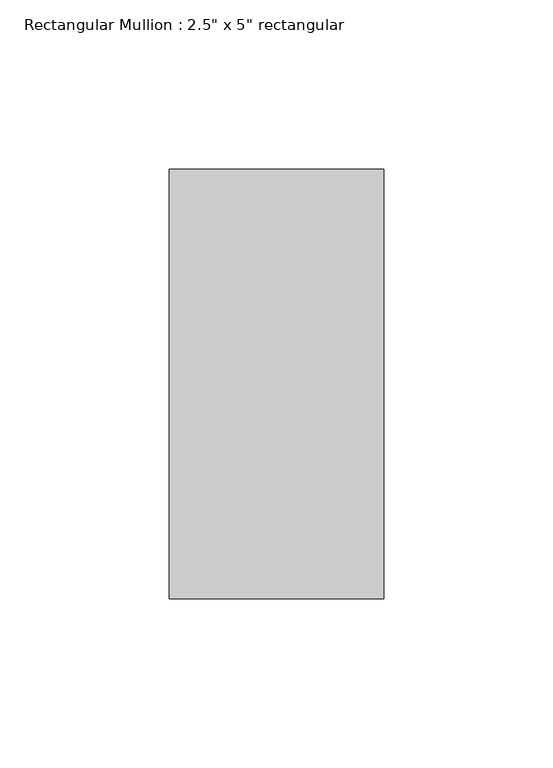
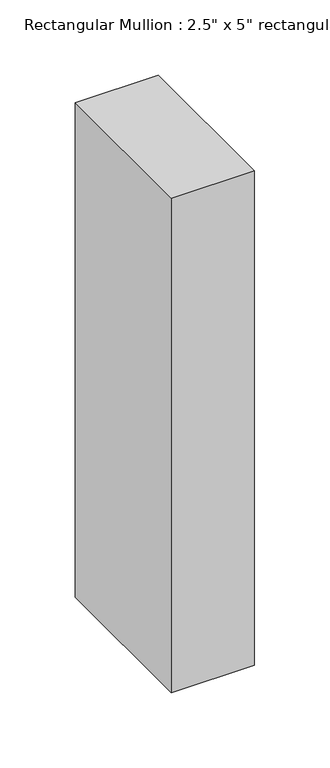
"""IFC4 building model written with IfcOpenShell, lengths in millimetres: member geometry."""

from ifc_helpers import new_model, si_unit, frame, origin, place, context, project, spatial, polyline, outline, extrude, source, transform, mapped, element, save


def member_d2340509(model_context):
    return source(origin(), model_context, "Body", "SweptSolid", [
        extrude(outline(polyline([(31.75, 63.5), (31.75, -63.5), (-31.75, -63.5), (-31.75, 63.5), (31.75, 63.5)])), frame((0.0, 0.0, -400.05), z_axis=(0.0, 0.0, 1.0), x_axis=(1.0, 0.0, 0.0)), (0.0, 0.0, 1.0), 400.05),
    ])


if __name__ == "__main__":
    model = new_model("IFC4")
    model_context = context("Model", 3, world=origin())
    ifc_project = project(units=[si_unit("LENGTHUNIT", "METRE", prefix="MILLI")], contexts=[model_context])
    site = spatial("IfcSite", under=ifc_project)
    building = spatial("IfcBuilding", under=site)
    placement = place(None, origin())
    member_shape = member_d2340509(model_context)
    element("IfcMember", 1, ObjectType="Rectangular Mullion : 2.5\" x 5\" rectangular", at=placement, inside=building, context=model_context, shape_type="MappedRepresentation", body=[
        mapped(member_shape, transform((0.0, 0.0, 0.0), x_axis=(1.0, 0.0, 0.0), y_axis=(0.0, 1.0, 0.0), z_axis=(0.0, 0.0, 1.0))),
    ])
    save(model, "model.ifc")

# Revit data of these elements
# Type "Rectangular Mullion : 2.5\" x 5\" rectangular"
#   built-in parameter 1007304 = 0.416667 (stored number, unit not read)
#   built-in parameter 1007301 = 0.104167 (stored number, unit not read)
#   built-in parameter 1007300 = 0.104167 (stored number, unit not read)
